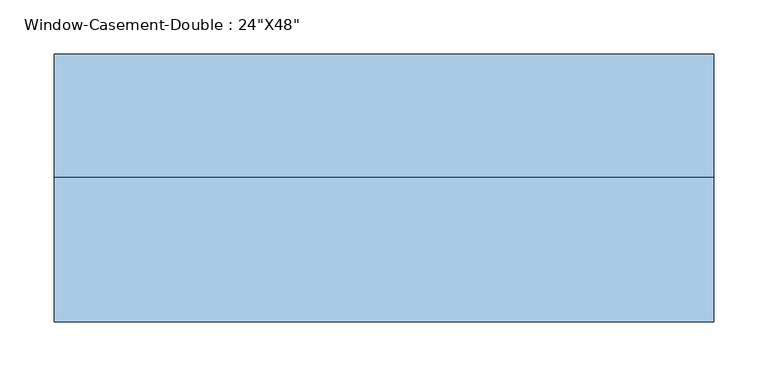
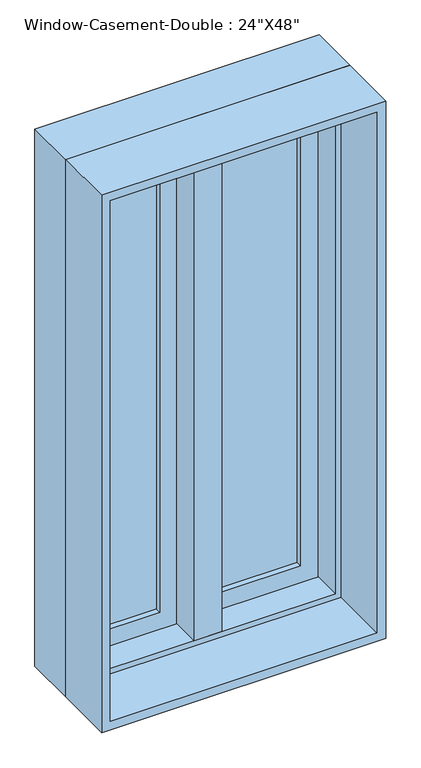
"""IFC4 building model written with IfcOpenShell, lengths in millimetres: window geometry."""

from ifc_helpers import new_model, si_unit, frame, origin, place, context, project, spatial, polyline, outline, extrude, faceted_brep, source, transform, mapped, element, save


def window_782a76c6(model_context):
    return source(origin(), model_context, "Body", "SolidModel", [
        faceted_brep([(9.525, 133.35, 2120.9), (-9.525, 133.35, 2120.9), (-9.525, 82.55, 2120.9), (9.525, 82.55, 2120.9), (9.525, 133.35, 927.1), (9.525, 82.55, 927.1), (-9.525, 82.55, 927.1), (-9.525, 133.35, 927.1), (-9.525, 82.55, 946.15), (-9.525, 82.55, 2101.85), (-30.1625, 82.55, 946.15), (-30.1625, 82.55, 2101.85), (-30.1625, 19.05, 946.15), (-30.1625, 19.05, 2101.85), (30.1625, 19.05, 946.15), (30.1625, 19.05, 2101.85), (30.1625, 82.55, 946.15), (30.1625, 82.55, 2101.85), (9.525, 82.55, 946.15), (9.525, 82.55, 2101.85)], [[[0, 1, 2, 3]], [[4, 5, 6, 7]], [[1, 0, 4, 7]], [[2, 1, 7, 6, 8, 9]], [[9, 8, 10, 11]], [[11, 10, 12, 13]], [[13, 12, 14, 15]], [[15, 14, 16, 17]], [[17, 16, 18, 19]], [[0, 3, 19, 18, 5, 4]], [[18, 8, 6, 5]], [[9, 19, 3, 2]], [[8, 18, 16, 14, 12, 10]], [[19, 9, 11, 13, 15, 17]]]),
        extrude(outline(polyline([(-66.675, 114.3), (-66.675, 107.95), (-234.95, 107.95), (-234.95, 114.3), (-66.675, 114.3)])), frame((0.0, 0.0, 984.25), z_axis=(0.0, 0.0, 1.0), x_axis=(1.0, 0.0, 0.0)), (0.0, 0.0, 1.0), 1079.5),
        extrude(outline(polyline([(-234.95, 95.25), (-234.95, 101.6), (-66.675, 101.6), (-66.675, 95.25), (-234.95, 95.25)])), frame((0.0, 0.0, 984.25), z_axis=(0.0, 0.0, 1.0), x_axis=(1.0, 0.0, 0.0)), (0.0, 0.0, 1.0), 1079.5),
        extrude(outline(polyline([(234.95, 114.3), (234.95, 107.95), (66.675, 107.95), (66.675, 114.3), (234.95, 114.3)])), frame((0.0, 0.0, 984.25), z_axis=(0.0, 0.0, 1.0), x_axis=(1.0, 0.0, 0.0)), (0.0, 0.0, 1.0), 1079.5),
        extrude(outline(polyline([(66.675, 95.25), (66.675, 101.6), (234.95, 101.6), (234.95, 95.25), (66.675, 95.25)])), frame((0.0, 0.0, 984.25), z_axis=(0.0, 0.0, 1.0), x_axis=(1.0, 0.0, 0.0)), (0.0, 0.0, 1.0), 1079.5),
        extrude(outline(polyline([(2120.9, -292.1), (927.1, -292.1), (927.1, -9.525), (2120.9, -9.525), (2120.9, -292.1)]), holes=[polyline([(2063.75, -66.675), (984.25, -66.675), (984.25, -234.95), (2063.75, -234.95), (2063.75, -66.675)])]), frame((0.0, 82.55, 0.0), z_axis=(0.0, 1.0, 0.0), x_axis=(0.0, 0.0, 1.0)), (0.0, 0.0, 1.0), 44.45),
        extrude(outline(polyline([(927.1, 292.1), (2120.9, 292.1), (2120.9, 9.525), (927.1, 9.525), (927.1, 292.1)]), holes=[polyline([(984.25, 66.675), (2063.75, 66.675), (2063.75, 234.95), (984.25, 234.95), (984.25, 66.675)])]), frame((0.0, 82.55, 0.0), z_axis=(0.0, 1.0, 0.0), x_axis=(0.0, 0.0, 1.0)), (0.0, 0.0, 1.0), 44.45),
        extrude(outline(polyline([(2133.6, -304.8), (914.4, -304.8), (914.4, 304.8), (2133.6, 304.8), (2133.6, -304.8)]), holes=[polyline([(2114.55, 285.75), (933.45, 285.75), (933.45, -285.75), (2114.55, -285.75), (2114.55, 285.75)])]), frame((0.0, -114.3, 0.0), z_axis=(0.0, 1.0, 0.0), x_axis=(0.0, 0.0, 1.0)), (0.0, 0.0, 1.0), 133.35),
        faceted_brep([(273.05, 82.55, 2101.85), (273.05, 19.05, 2101.85), (-273.05, 19.05, 2101.85), (-273.05, 82.55, 2101.85), (292.1, 133.35, 2120.9), (292.1, 82.55, 2120.9), (-292.1, 82.55, 2120.9), (-292.1, 133.35, 2120.9), (304.8, 19.05, 2133.6), (304.8, 133.35, 2133.6), (-304.8, 133.35, 2133.6), (-304.8, 19.05, 2133.6), (-273.05, 19.05, 946.15), (-273.05, 82.55, 946.15), (-292.1, 82.55, 927.1), (-292.1, 133.35, 927.1), (-304.8, 133.35, 914.4), (-304.8, 19.05, 914.4), (273.05, 19.05, 946.15), (273.05, 82.55, 946.15), (292.1, 82.55, 927.1), (292.1, 133.35, 927.1), (304.8, 133.35, 914.4), (304.8, 19.05, 914.4)], [[[0, 1, 2, 3]], [[4, 5, 6, 7]], [[8, 9, 10, 11]], [[3, 2, 12, 13]], [[7, 6, 14, 15]], [[11, 10, 16, 17]], [[13, 12, 18, 19]], [[15, 14, 20, 21]], [[17, 16, 22, 23]], [[11, 17, 23, 8], [1, 18, 12, 2]], [[19, 18, 1, 0]], [[5, 20, 14, 6], [3, 13, 19, 0]], [[21, 20, 5, 4]], [[23, 22, 9, 8]], [[9, 22, 16, 10], [7, 15, 21, 4]]]),
    ])


if __name__ == "__main__":
    model = new_model("IFC4")
    model_context = context("Model", 3, world=origin())
    ifc_project = project(units=[si_unit("LENGTHUNIT", "METRE", prefix="MILLI")], contexts=[model_context])
    site = spatial("IfcSite", under=ifc_project)
    building = spatial("IfcBuilding", under=site)
    placement = place(None, origin())
    window_shape = window_782a76c6(model_context)
    element("IfcWindow", 1, ObjectType="Window-Casement-Double : 24\"X48\"", at=placement, inside=building, context=model_context, shape_type="MappedRepresentation", body=[
        mapped(window_shape, transform((0.0, 0.0, 0.0), x_axis=(1.0, 0.0, 0.0), y_axis=(0.0, 1.0, 0.0), z_axis=(0.0, 0.0, 1.0))),
    ])
    save(model, "model.ifc")

# Revit data of these elements
# Type "Window-Casement-Double : 24\"X48\""
#   Type Mark = "22"
#   Fire Rating = "0.5h"
#   Assembly Code = "B2020100"
#   Analytic Construction = "Double glazing - domestic"
#   Frame Extension [instance default] = 0' - 0 1/4"
#   Window Inset [instance default] = 0' - 0"
#   Wall Thickness [instance default] = 0' - 6"
#   Interior Wall Closure [instance default] = 0' - 2 1/4"
#   Half Width = 1' - 0"
#   Visual Light Transmittance = 0.81
#   Thermal Resistance (R) = 1.8146 (h·ft²·°F)/BTU
#   Solar Heat Gain Coefficient = 0.76
#   Rough Width = 2' - 0 1/2"
#   Rough Height = 4' - 0 1/2"
#   Height = 4' - 0"
#   Heat Transfer Coefficient (U) = 0.5511 BTU/(h·ft²·°F)
#   Exterior Wall Closure [instance default] = 0' - 1 1/4"
#   Extension Jamb [instance default] = 0' - 2 1/4"
#   Default Sill Height = 3' - 0"
#   Width = 2' - 0"
#   Muntin Visibility = yes
#   Interior Trim Visibility [instance default] = yes
#   Exterior Trim Visibility [instance default] = yes
#   Extension Jamb Visibility [instance default] = yes
#   Interior Trim Material = Wood - Stained
#   Muntin Pattern = Muntin Pattern_2x2 : Muntin Pattern_2x2
#   Interior Trim = Trim-Window-Interior-Flat : Picture Frame
#   Interior Frame Material = Wood - Stained
#   Glass Panel Material = Glass
#   Exterior Trim Material = Clad - White
#   Exterior Trim = Trim-Window-Exterior-Flat : with Sill
#   Exterior Frame Material = Clad - White
#   Wall Closure = (empty or 0)
# Element 1 (IfcWindow, "Window-Casement-Double : 24\"X48\"")
#   Wall Thickness = 0' - 9"
#   Extension Jamb = 0' - 5 1/4"
#   Materials on its faces: "Wood - Stained", "Glass", "Clad - White"
# Materials
#   "Wood - Stained": class "Wood", colour RGB 224 178 126, transparency 0, Cost = 0
#   "Glass": class "Glass", colour RGB 0 128 192, transparency 0.75, Description = "Soda Lime Glass", Cost = 0
#   "Clad - White": class "Wood", colour RGB 242 242 238, transparency 0, Cost = 0
